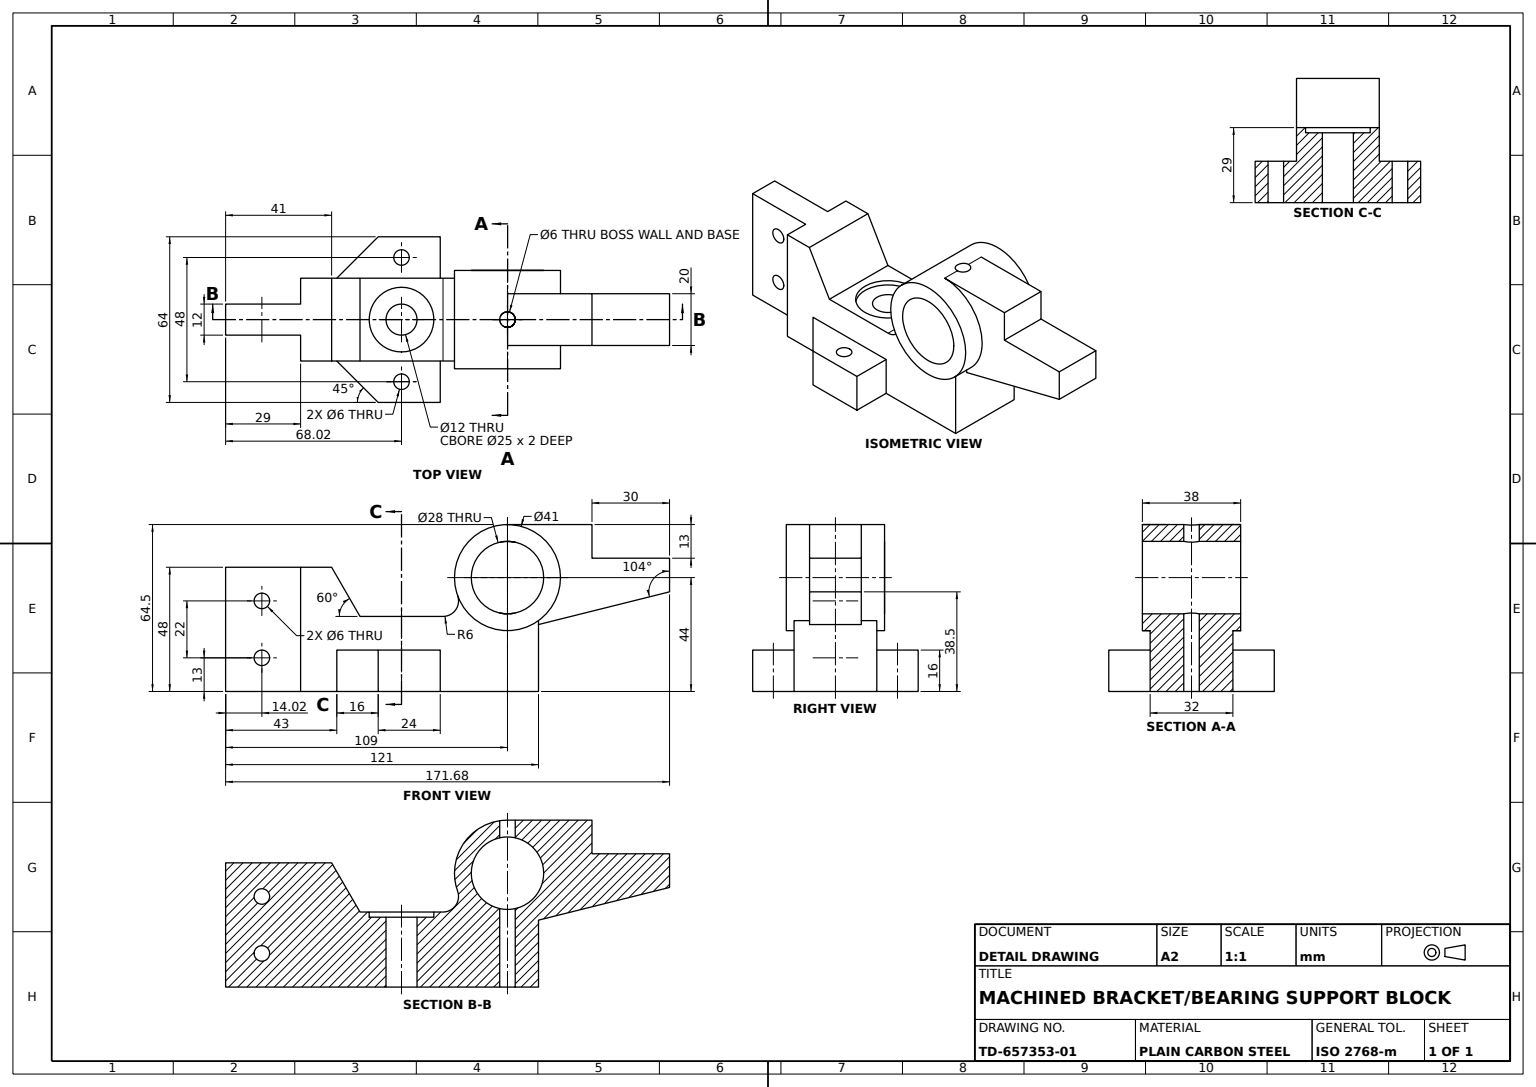
from build123d import *

# Parameters (mm, degrees)
BASE_BLOCK_SKETCH_W                = 121
BASE_BLOCK_SKETCH_H                = 48
BASE_BLOCK_121X48_DEPTH            = 16
BASE_STEP_SKETCH_W                 = 10
BASE_STEP_SKETCH_H                 = 48
BASE_STEP_CUT_DEPTH                = 29
ANGLED_RELIEF_CUT_30DEG_DEPTH      = 73.527580961
ANGLED_RELIEF_CUT_30DEG_DEPTH_BACK = 73.527580961
PIVOT_BOSS_SKETCH_R                = 20.5
PIVOT_BOSS_44_DEPTH                = 19
PIVOT_BOSS_FILLET_R6_R             = 6
CLAMP_TAB_DEPTH                    = 10
TAB_PIN_HOLE_6_DEPTH               = 120.841457826
TAB_PIN_HOLE_6_DEPTH_BACK          = 120.841457826
TAB_PIN_HOLE_SKETCH_R              = 3
PIVOT_BORE_28_DEPTH                = 125.277813908
PIVOT_BORE_28_DEPTH_BACK           = 125.277813908
PIVOT_BORE_SKETCH_R                = 14
COUNTERBORED_HOLE_12_D             = 12
COUNTERBORED_HOLE_12_CBORE_D       = 25
COUNTERBORED_HOLE_12_CBORE_DEPTH   = 2
MOUNTING_FLANGE_SKETCH_R           = 3
MOUNTING_FLANGE_DEPTH              = 16
END_SLOT_CUT_DEPTH                 = 125.277813877
END_SLOT_CUT_DEPTH_BACK            = 125.277813877
END_SLOT_SKETCH_R                  = 3


with BuildPart() as part:
    # Base Block Sketch → Base Block 121x48 (new, symmetric)
    with BuildSketch(Plane.XY):
        Rectangle(BASE_BLOCK_SKETCH_W, BASE_BLOCK_SKETCH_H)
    extrude(amount=BASE_BLOCK_121X48_DEPTH, both=True)

    # Base Step Sketch → Base Step Cut (cut)
    with BuildSketch(Plane(origin=(60.5, 0, 0), x_dir=(0, 0, -1), z_dir=(1, 0, 0))):
        with Locations((-11, 0)):
            Rectangle(BASE_STEP_SKETCH_W, BASE_STEP_SKETCH_H)
        with Locations((11, 0)):
            Rectangle(BASE_STEP_SKETCH_W, BASE_STEP_SKETCH_H)
    extrude(amount=-BASE_STEP_CUT_DEPTH, mode=Mode.SUBTRACT)

    # Angled Relief Sketch → Angled Relief Cut 30deg (cut, two sides: drawn at the far end of the back side and taken through both)
    with BuildSketch(Plane.XY.offset(16).offset(-ANGLED_RELIEF_CUT_30DEG_DEPTH_BACK)):
        Polygon((19.5, 24), (8.530344885, 5), (-40, 5), (-40, 24), align=None)
    extrude(amount=ANGLED_RELIEF_CUT_30DEG_DEPTH + ANGLED_RELIEF_CUT_30DEG_DEPTH_BACK, mode=Mode.SUBTRACT)

    # Pivot Boss Sketch → Pivot Boss Ø44 (add, symmetric)
    with BuildSketch(Plane.XY):
        with Locations((-48.5, 20)):
            Circle(PIVOT_BOSS_SKETCH_R)
    extrude(amount=PIVOT_BOSS_44_DEPTH, both=True)

    # Pivot Boss Fillet R6
    pivot_boss_fillet_r6_edges = [part.edges().sort_by_distance(p)[0] for p in [
        (-34.526811388, 5, 0),
    ]]
    fillet(pivot_boss_fillet_r6_edges, radius=PIVOT_BOSS_FILLET_R6_R)

    # Clamp Tab Sketch → Clamp Tab (add, symmetric)
    with BuildSketch(Plane.XY):
        with BuildLine():
            Line((-48.5, 40.5), (-81.178797502, 40.5))
            Line((-81.178797502, 40.5), (-81.178797502, 27.5))
            Line((-81.178797502, 27.5), (-111.178797502, 27.5))
            Line((-111.178797502, 27.5), (-111.178797502, 14.5))
            Line((-111.178797502, 14.5), (-53.45939886, 0.108937611))
            ThreePointArc((-53.45939886, 0.108937611), (-68.847196109, 22.49832154), (-48.5, 40.5))
        make_face()
    extrude(amount=CLAMP_TAB_DEPTH, both=True)

    # Tab Pin Hole Sketch → Tab Pin Hole Ø6 (cut, two sides: drawn at the far end of the back side and taken through both)
    with BuildSketch(Plane(origin=(0, 0, 0), x_dir=(1, 0, 0), z_dir=(0, 1, 0)).offset(-TAB_PIN_HOLE_6_DEPTH_BACK)):
        with Locations(Location((-48.5, 0, 0), (0, 0, 270))):
            Circle(TAB_PIN_HOLE_SKETCH_R)
    extrude(amount=TAB_PIN_HOLE_6_DEPTH + TAB_PIN_HOLE_6_DEPTH_BACK, mode=Mode.SUBTRACT)

    # Pivot Bore Sketch → Pivot Bore Ø28 (cut, two sides: drawn at the far end of the back side and taken through both)
    with BuildSketch(Plane.XY.offset(19).offset(-PIVOT_BORE_28_DEPTH_BACK)):
        with Locations((-48.5, 20)):
            Circle(PIVOT_BORE_SKETCH_R)
    extrude(amount=PIVOT_BORE_28_DEPTH + PIVOT_BORE_28_DEPTH_BACK, mode=Mode.SUBTRACT)

    # Counterbored Hole Ø12 (through all)
    with Locations(Plane(origin=(0, 5, 0), x_dir=(1, 0, 0), z_dir=(0, 1, 0))):
        with Locations((-7.522383977, 0)):
            CounterBoreHole(COUNTERBORED_HOLE_12_D / 2, COUNTERBORED_HOLE_12_CBORE_D / 2, COUNTERBORED_HOLE_12_CBORE_DEPTH)

    # Mounting Flange Sketch → Mounting Flange (add)
    # profile 1 of 2: a face of its own
    with BuildSketch(Plane.XZ.offset(24)):
        Polygon((-22.5, -16), (-22.5, -32), (1.5, -32), (17.5, -16), align=None)
        with Locations(Location((-7.522383977, -24, 0), (0, 0, 270))):
            Circle(MOUNTING_FLANGE_SKETCH_R, mode=Mode.SUBTRACT)
    # profile 2 of 2: a face of its own
    with BuildSketch(Plane.XZ.offset(24)):
        Polygon((17.5, 16), (-22.5, 16), (-22.5, 32), (1.5, 32), align=None)
        with Locations(Location((-7.522383977, 24, 0), (0, 0, 270))):
            Circle(MOUNTING_FLANGE_SKETCH_R, mode=Mode.SUBTRACT)
    extrude(amount=-MOUNTING_FLANGE_DEPTH)

    # End Slot Sketch → End Slot Cut (cut, two sides: drawn at the far end of the back side and taken through both)
    with BuildSketch(Plane.XY.offset(6).offset(-END_SLOT_CUT_DEPTH_BACK)):
        with Locations((46.48, 11)):
            Circle(END_SLOT_SKETCH_R)
        with Locations((46.48, -11)):
            Circle(END_SLOT_SKETCH_R)
    extrude(amount=END_SLOT_CUT_DEPTH + END_SLOT_CUT_DEPTH_BACK, mode=Mode.SUBTRACT)


solid = part.part
